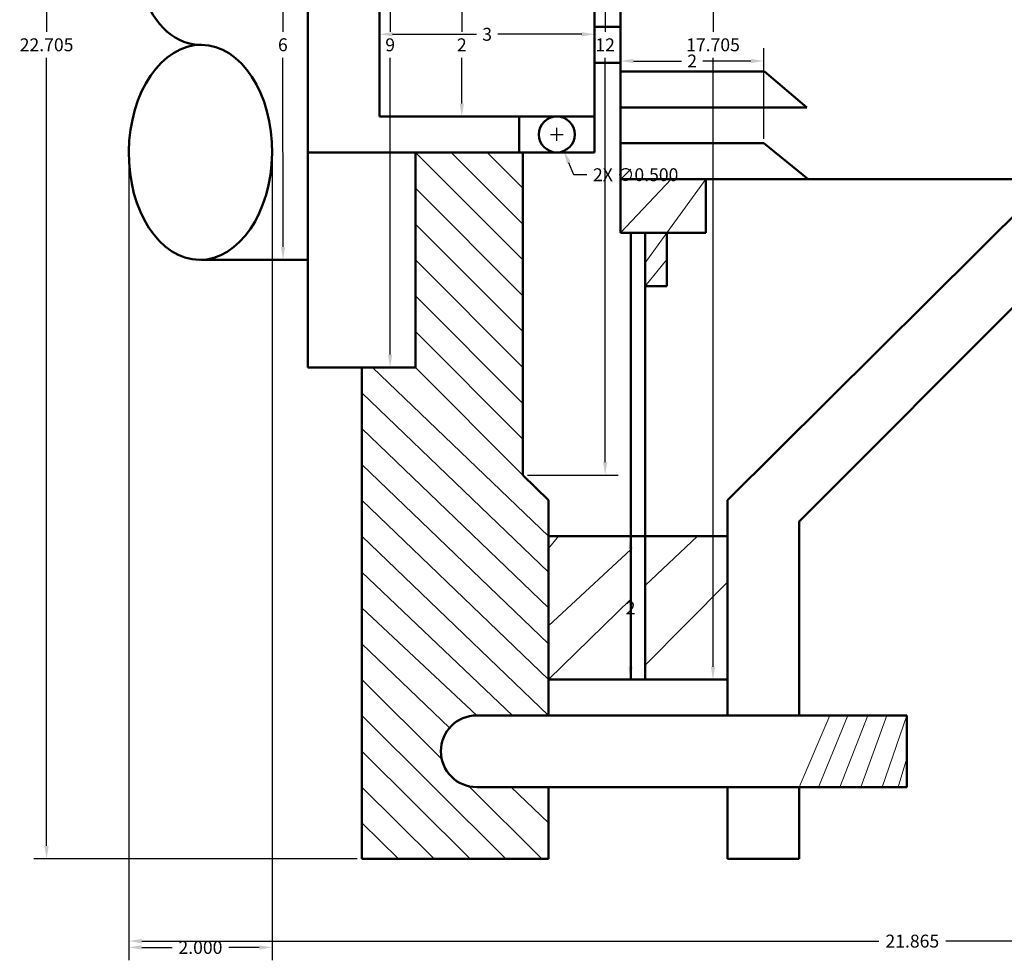
# Model space of a CAD drawing. Units: inches. Extents: x 15.4 to 41.1, y -0.4 to 25.1.
# Tile 1 of 4: x 16 to 29.7, y -0.4 to 12.7. Entities that reach past the tile are written whole.
import ezdxf

# ---------------------------------------------------------------- set-up
doc = ezdxf.new("R2010")
doc.units = ezdxf.units.IN
doc.header["$MEASUREMENT"] = 0
for name, color, linetype, lineweight in [('M-DIMS', 2, 'Continuous', 18), ('M-HATC', 8, 'Continuous', 18), ('M-OUTL', 7, 'Continuous', 50)]:
    doc.layers.add(name, color=color, linetype=linetype, lineweight=lineweight)
doc.styles.get("Standard").update_dxf_attribs({"font": 'arial.ttf'})
doc.dimstyles.get("Standard").update_dxf_attribs({"dimtxt": 0.18, "dimasz": 0.18, "dimexe": 0.18, "dimexo": 0.0625, "dimgap": 0.09, "dimtad": 0, "dimtih": 1, "dimtoh": 1, "dimdec": 4, "dimzin": 0, "dimdsep": 46, "dimtxsty": 'Standard', "dimcen": 0.09, "dimadec": 0, "dimazin": 0, "dimtfac": 1, "dimtdec": 4, "dimtofl": 0, "dimtmove": 0, "dimatfit": 3, "dimfxl": 1, "dimtolj": 1, "dimtzin": 0, "dimarcsym": 0})

# ---------------------------------------------------------------- blocks, each defined once
blk = doc.blocks.new('*D1')
at = {"layer": 'Defpoints', "color": 0, "transparency": 16777216}
for p in [(39.379, 12.649), (17.513, 10.885), (39.379, -0.125)]:
    blk.add_point(p, dxfattribs=at)
at = {"layer": 'M-DIMS', "color": 0, "lineweight": -2, "transparency": 16777216}
for p, q in [((39.379, 12.587), (39.379, -0.305)), ((17.513, 10.823), (17.513, -0.305)), ((17.693, -0.125), (27.98, -0.125)), ((39.199, -0.125), (28.912, -0.125))]:
    blk.add_line(p, q, dxfattribs=at)
at = {"layer": 'M-DIMS', "color": 0, "transparency": 16777216}
for points in [[(17.693, -0.095), (17.693, -0.155), (17.513, -0.125)], [(39.199, -0.095), (39.199, -0.155), (39.379, -0.125)]]:
    blk.add_solid(points, dxfattribs=at)
at = {"layer": 'M-DIMS', "color": 0, "transparency": 16777216, "insert": (28.446, -0.125), "char_height": 0.18, "attachment_point": 5}
blk.add_mtext('\\A1;21.865', dxfattribs=at)
blk = doc.blocks.new('*D2')
at = {"layer": 'Defpoints', "color": 0, "transparency": 16777216}
for p in [(16.366, 23.727), (20.763, 23.727), (20.763, 1.022)]:
    blk.add_point(p, dxfattribs=at)
at = {"layer": 'M-DIMS', "color": 0, "lineweight": -2, "transparency": 16777216}
for p, q in [((20.7, 23.727), (16.186, 23.727)), ((16.366, 23.547), (16.366, 12.557)), ((16.366, 1.202), (16.366, 12.193)), ((20.7, 1.022), (16.186, 1.022))]:
    blk.add_line(p, q, dxfattribs=at)
at = {"layer": 'M-DIMS', "color": 0, "transparency": 16777216}
for points in [[(16.336, 23.547), (16.396, 23.547), (16.366, 23.727)], [(16.336, 1.202), (16.396, 1.202), (16.366, 1.022)]]:
    blk.add_solid(points, dxfattribs=at)
at = {"layer": 'M-DIMS', "color": 0, "transparency": 16777216, "insert": (16.366, 12.375), "char_height": 0.18, "attachment_point": 5}
blk.add_mtext('\\A1;22.705', dxfattribs=at)
blk = doc.blocks.new('*D17')
at = {"layer": 'Defpoints', "color": 0, "transparency": 16777216}
for p in [(23.368, 5.522), (23.368, 3.522), (24.515, 3.522)]:
    blk.add_point(p, dxfattribs=at)
at = {"layer": 'M-DIMS', "color": 0, "lineweight": -2, "transparency": 16777216}
for p, q in [((23.43, 5.522), (24.695, 5.522)), ((24.515, 5.342), (24.515, 4.703)), ((24.515, 3.702), (24.515, 4.342)), ((23.43, 3.522), (24.695, 3.522))]:
    blk.add_line(p, q, dxfattribs=at)
at = {"layer": 'M-DIMS', "color": 0, "transparency": 16777216}
for points in [[(24.485, 5.342), (24.545, 5.342), (24.515, 5.522)], [(24.485, 3.702), (24.545, 3.702), (24.515, 3.522)]]:
    blk.add_solid(points, dxfattribs=at)
at = {"layer": 'M-DIMS', "color": 0, "transparency": 16777216, "insert": (24.515, 4.522), "char_height": 0.18, "attachment_point": 5}
blk.add_mtext('\\A1;2', dxfattribs=at)
blk = doc.blocks.new('*D18')
at = {"layer": 'Defpoints', "color": 0, "transparency": 16777216}
for p in [(24.518, 21.227), (24.518, 3.522), (25.665, 3.522)]:
    blk.add_point(p, dxfattribs=at)
at = {"layer": 'M-DIMS', "color": 0, "lineweight": -2, "transparency": 16777216}
for p, q in [((24.58, 21.227), (25.845, 21.227)), ((25.665, 21.047), (25.665, 12.557)), ((25.665, 3.702), (25.665, 12.193)), ((24.58, 3.522), (25.845, 3.522))]:
    blk.add_line(p, q, dxfattribs=at)
at = {"layer": 'M-DIMS', "color": 0, "transparency": 16777216}
for points in [[(25.635, 21.047), (25.695, 21.047), (25.665, 21.227)], [(25.635, 3.702), (25.695, 3.702), (25.665, 3.522)]]:
    blk.add_solid(points, dxfattribs=at)
at = {"layer": 'M-DIMS', "color": 0, "transparency": 16777216, "insert": (25.665, 12.375), "char_height": 0.18, "attachment_point": 5}
blk.add_mtext('\\A1;17.705', dxfattribs=at)
blk = doc.blocks.new('*D19')
at = {"layer": 'Defpoints', "color": 0, "transparency": 16777216}
for p in [(23.013, 18.375), (23.013, 6.375), (24.16, 6.375)]:
    blk.add_point(p, dxfattribs=at)
at = {"layer": 'M-DIMS', "color": 0, "lineweight": -2, "transparency": 16777216}
for p, q in [((23.075, 18.375), (24.34, 18.375)), ((24.16, 18.195), (24.16, 12.555)), ((24.16, 6.555), (24.16, 12.194)), ((23.075, 6.375), (24.34, 6.375))]:
    blk.add_line(p, q, dxfattribs=at)
at = {"layer": 'M-DIMS', "color": 0, "transparency": 16777216}
for points in [[(24.13, 18.195), (24.19, 18.195), (24.16, 18.375)], [(24.13, 6.555), (24.19, 6.555), (24.16, 6.375)]]:
    blk.add_solid(points, dxfattribs=at)
at = {"layer": 'M-DIMS', "color": 0, "transparency": 16777216, "insert": (24.16, 12.375), "char_height": 0.18, "attachment_point": 5}
blk.add_mtext('\\A1;12', dxfattribs=at)
blk = doc.blocks.new('*D21')
at = {"layer": 'Defpoints', "color": 0, "transparency": 16777216}
for p in [(20.013, 16.875), (20.013, 7.875), (21.16, 7.875)]:
    blk.add_point(p, dxfattribs=at)
at = {"layer": 'M-DIMS', "color": 0, "lineweight": -2, "transparency": 16777216}
for p, q in [((20.075, 16.875), (21.34, 16.875)), ((21.16, 16.695), (21.16, 12.557)), ((21.16, 8.055), (21.16, 12.193)), ((20.075, 7.875), (21.34, 7.875))]:
    blk.add_line(p, q, dxfattribs=at)
at = {"layer": 'M-DIMS', "color": 0, "transparency": 16777216}
for points in [[(21.13, 16.695), (21.19, 16.695), (21.16, 16.875)], [(21.13, 8.055), (21.19, 8.055), (21.16, 7.875)]]:
    blk.add_solid(points, dxfattribs=at)
at = {"layer": 'M-DIMS', "color": 0, "transparency": 16777216, "insert": (21.16, 12.375), "char_height": 0.18, "attachment_point": 5}
blk.add_mtext('\\A1;9', dxfattribs=at)
blk = doc.blocks.new('*D23')
at = {"layer": 'Defpoints', "color": 0, "transparency": 16777216}
for p in [(18.513, 15.375), (18.518, 9.375), (19.665, 9.376)]:
    blk.add_point(p, dxfattribs=at)
at = {"layer": 'M-DIMS', "color": 0, "lineweight": -2, "transparency": 16777216}
for p, q in [((18.575, 15.375), (19.84, 15.376)), ((19.66, 15.196), (19.663, 12.558)), ((19.665, 9.556), (19.663, 12.194)), ((18.58, 9.375), (19.845, 9.376))]:
    blk.add_line(p, q, dxfattribs=at)
at = {"layer": 'M-DIMS', "color": 0, "transparency": 16777216}
for points in [[(19.69, 15.196), (19.63, 15.196), (19.66, 15.376)], [(19.695, 9.556), (19.635, 9.556), (19.665, 9.376)]]:
    blk.add_solid(points, dxfattribs=at)
at = {"layer": 'M-DIMS', "color": 0, "transparency": 16777216, "insert": (19.663, 12.376), "char_height": 0.18, "attachment_point": 5}
blk.add_mtext('\\A1;6', dxfattribs=at)
blk = doc.blocks.new('*D24')
at = {"layer": 'Defpoints', "color": 0, "transparency": 16777216}
for p in [(21.013, 13.375), (21.013, 11.375), (22.16, 11.375)]:
    blk.add_point(p, dxfattribs=at)
at = {"layer": 'M-DIMS', "color": 0, "lineweight": -2, "transparency": 16777216}
for p, q in [((21.075, 13.375), (22.34, 13.375)), ((22.16, 13.195), (22.16, 12.555)), ((22.16, 11.555), (22.16, 12.194)), ((21.075, 11.375), (22.34, 11.375))]:
    blk.add_line(p, q, dxfattribs=at)
at = {"layer": 'M-DIMS', "color": 0, "transparency": 16777216}
for points in [[(22.13, 13.195), (22.19, 13.195), (22.16, 13.375)], [(22.13, 11.555), (22.19, 11.555), (22.16, 11.375)]]:
    blk.add_solid(points, dxfattribs=at)
at = {"layer": 'M-DIMS', "color": 0, "transparency": 16777216, "insert": (22.16, 12.375), "char_height": 0.18, "attachment_point": 5}
blk.add_mtext('\\A1;2', dxfattribs=at)
blk = doc.blocks.new('*D25')
at = {"layer": 'Defpoints', "color": 0, "transparency": 16777216}
for p in [(24.013, 12.522), (21.013, 11.375), (24.013, 11.375)]:
    blk.add_point(p, dxfattribs=at)
at = {"layer": 'M-DIMS', "color": 0, "lineweight": -2, "transparency": 16777216}
for p, q in [((21.013, 11.437), (21.013, 12.702)), ((24.013, 11.437), (24.013, 12.702)), ((21.193, 12.522), (22.364, 12.522)), ((23.833, 12.522), (22.662, 12.522))]:
    blk.add_line(p, q, dxfattribs=at)
at = {"layer": 'M-DIMS', "color": 0, "transparency": 16777216}
for points in [[(21.193, 12.552), (21.193, 12.492), (21.013, 12.522)], [(23.833, 12.552), (23.833, 12.492), (24.013, 12.522)]]:
    blk.add_solid(points, dxfattribs=at)
at = {"layer": 'M-DIMS', "color": 0, "transparency": 16777216, "insert": (22.513, 12.522), "char_height": 0.18, "attachment_point": 5}
blk.add_mtext('\\A1;3', dxfattribs=at)
blk = doc.blocks.new('*D30')
at = {"layer": 'Defpoints', "color": 0, "transparency": 16777216}
for p in [(26.374, 12.149), (24.374, 11.001), (26.374, 11.001)]:
    blk.add_point(p, dxfattribs=at)
at = {"layer": 'M-DIMS', "color": 0, "lineweight": -2, "transparency": 16777216}
for p, q in [((24.374, 11.064), (24.374, 12.329)), ((26.374, 11.064), (26.374, 12.329)), ((24.554, 12.149), (25.224, 12.149)), ((26.194, 12.149), (25.524, 12.149))]:
    blk.add_line(p, q, dxfattribs=at)
at = {"layer": 'M-DIMS', "color": 0, "transparency": 16777216}
for points in [[(24.554, 12.179), (24.554, 12.119), (24.374, 12.149)], [(26.194, 12.179), (26.194, 12.119), (26.374, 12.149)]]:
    blk.add_solid(points, dxfattribs=at)
at = {"layer": 'M-DIMS', "color": 0, "transparency": 16777216, "insert": (25.374, 12.149), "char_height": 0.18, "attachment_point": 5}
blk.add_mtext('\\A1;2', dxfattribs=at)
blk = doc.blocks.new('*D50')
at = {"layer": 'Defpoints', "color": 0, "transparency": 16777216}
for p in [(17.513, 10.885), (19.513, 10.864), (19.513, -0.213)]:
    blk.add_point(p, dxfattribs=at)
at = {"layer": 'M-DIMS', "color": 0, "lineweight": -2, "transparency": 16777216}
for p, q in [((17.513, 10.823), (17.513, -0.393)), ((19.513, 10.802), (19.513, -0.393)), ((17.693, -0.213), (18.118, -0.213)), ((19.333, -0.213), (18.908, -0.213))]:
    blk.add_line(p, q, dxfattribs=at)
at = {"layer": 'M-DIMS', "color": 0, "transparency": 16777216}
for points in [[(17.693, -0.183), (17.693, -0.243), (17.513, -0.213)], [(19.333, -0.183), (19.333, -0.243), (19.513, -0.213)]]:
    blk.add_solid(points, dxfattribs=at)
at = {"layer": 'M-DIMS', "color": 0, "transparency": 16777216, "insert": (18.513, -0.213), "char_height": 0.18, "attachment_point": 5}
blk.add_mtext('\\A1;2.000', dxfattribs=at)
blk = doc.blocks.new('*D60')
at = {"layer": 'Defpoints', "color": 0, "transparency": 16777216}
for p in [(23.388, 11.355), (23.584, 10.895)]:
    blk.add_point(p, dxfattribs=at)
at = {"layer": 'M-DIMS', "color": 0, "lineweight": -2, "transparency": 16777216}
for p, q in [((23.486, 11.035), (23.486, 11.215)), ((23.396, 11.125), (23.576, 11.125)), ((23.724, 10.563), (23.654, 10.729)), ((23.904, 10.563), (23.724, 10.563))]:
    blk.add_line(p, q, dxfattribs=at)
at = {"layer": 'M-DIMS', "color": 0, "transparency": 16777216}
blk.add_solid([(23.681, 10.741), (23.626, 10.717), (23.584, 10.895)], dxfattribs=at)
at = {"layer": 'M-DIMS', "color": 0, "transparency": 16777216, "insert": (24.586, 10.563), "char_height": 0.18, "attachment_point": 5}
blk.add_mtext('\\A1;2X ∅0.500', dxfattribs=at)

msp = doc.modelspace()

# ---------------------------------------------------------------- linework, layer by layer
at = {"layer": 'M-HATC'}
for p, q in [((23.0128, 9.3747), (21.5128, 10.8747)), ((22.0128, 10.8747), (23.0128, 9.8747)), ((22.5128, 10.8747), (23.0128, 10.3747)), ((24.374, 9.7512), (25.0794, 10.5012)), ((25.5651, 10.5012), (25.0198, 9.7512)), ((21.5128, 10.3747), (23.0128, 8.8747)), ((23.0128, 8.3747), (21.5128, 9.8747)), ((25.0198, 9.7512), (24.7176, 9.3356)), ((21.5128, 9.3747), (23.0128, 7.8747)), ((24.7176, 9.0071), (25.0198, 9.3792)), ((23.0128, 7.3747), (21.5128, 8.8747)), ((21.5128, 8.3747), (23.0128, 6.8747)), ((20.9128, 7.8747), (23.3676, 5.5224)), ((23.0128, 6.3747), (21.5128, 7.8747)), ((23.3676, 5.0224), (20.7628, 7.5224)), ((23.3676, 4.5224), (20.7628, 7.0224)), ((20.7628, 6.5224), (23.3676, 4.0224)), ((23.3676, 3.5224), (20.7628, 6.0224)), ((20.7628, 5.5224), (23.3676, 3.0224)), ((23.3676, 5.3495), (23.5085, 5.5224)), ((24.7176, 4.833), (25.4478, 5.5224)), ((23.3676, 4.2724), (24.5176, 5.3372)), ((22.8676, 3.0224), (20.7628, 5.0224)), ((24.7176, 3.7238), (25.8676, 4.8821)), ((23.3676, 3.5224), (24.5176, 4.6441)), ((22.3676, 3.0224), (20.7628, 4.5224)), ((20.7628, 4.0224), (21.9874, 2.8471)), ((21.8801, 2.411), (20.7628, 3.5224)), ((20.7628, 3.0224), (22.7762, 1.0224)), ((26.8676, 2.0224), (27.2933, 3.0224)), ((27.5483, 3.0224), (27.1388, 2.0224)), ((27.4324, 2.0224), (27.8264, 3.0224)), ((28.0892, 3.0224), (27.726, 2.0224)), ((28.0274, 2.0224), (28.3676, 3.0224)), ((22.2762, 1.0224), (20.7628, 2.5224)), ((28.2467, 2.0224), (28.3676, 2.4241)), ((20.7628, 2.0224), (21.7762, 1.0224)), ((23.2762, 1.0224), (22.2588, 2.0344)), ((22.8466, 2.0224), (23.3676, 1.5224)), ((20.7628, 1.5224), (21.2762, 1.0224))]:
    msp.add_line(p, q, dxfattribs=at)
at = {"layer": 'M-OUTL'}
for p, q in [((24.374, 10.5012), (24.374, 14.5012)), ((24.374, 10.5012), (24.374, 14.5012)), ((24.374, 14.2482), (24.374, 10.2482)), ((24.374, 14.2482), (24.374, 10.2482)), ((20.0128, 12.3747), (20.0128, 13.8747)), ((24.0128, 13.8747), (24.0128, 10.8747)), ((24.0128, 10.8747), (24.0128, 13.8747)), ((21.0128, 13.3747), (21.0128, 11.3747)), ((21.0128, 11.3747), (21.0128, 13.3747)), ((24.0128, 12.3747), (24.0128, 12.6247)), ((24.0128, 12.6247), (24.374, 12.6247)), ((18.513, 12.3747), (18.513, 12.3745)), ((18.5287, 12.3746), (18.513, 12.3746)), ((18.5287, 12.3746), (18.5287, 12.3753)), ((20.0128, 10.8747), (20.0128, 12.3747)), ((20.0128, 12.3747), (20.0128, 10.8747)), ((24.0128, 12.3747), (24.0128, 12.1247)), ((24.0128, 12.1247), (24.374, 12.1247)), ((24.374, 11.5012), (24.374, 12.0012)), ((24.374, 12.0012), (26.3813, 12.0012)), ((24.374, 11.5012), (24.374, 12.0012)), ((24.374, 12.0012), (26.3813, 12.0012)), ((26.3813, 12.0012), (26.9763, 11.5012)), ((26.3813, 12.0012), (26.9763, 11.5012)), ((24.374, 11.0012), (24.374, 11.5012)), ((24.374, 11.5012), (26.9763, 11.5012)), ((24.374, 11.0012), (24.374, 11.5012)), ((24.374, 11.5012), (26.9763, 11.5012)), ((21.0128, 11.3747), (24.0128, 11.3747)), ((24.0128, 11.3747), (21.0128, 11.3747)), ((22.9588, 11.3747), (22.9588, 10.8747)), ((22.9588, 10.8747), (22.9588, 11.3747)), ((22.9588, 11.3747), (24.0128, 11.3747)), ((24.0128, 10.8747), (24.0128, 11.3747)), ((24.0128, 10.8747), (24.0128, 11.3747)), ((24.374, 10.5012), (24.374, 11.0012)), ((24.374, 11.0012), (26.374, 11.0012)), ((24.374, 10.5012), (24.374, 11.0012)), ((24.374, 11.0012), (26.374, 11.0012)), ((26.374, 11.0012), (26.9908, 10.5012)), ((26.374, 11.0012), (26.9908, 10.5012)), ((24.0128, 10.8747), (20.0128, 10.8747)), ((20.0128, 7.8747), (20.0128, 10.8747)), ((20.0128, 10.8747), (20.0128, 7.8747)), ((20.0128, 10.8747), (24.0128, 10.8747)), ((24.0128, 10.8747), (20.0128, 10.8747)), ((20.0128, 10.8747), (20.0128, 7.8747)), ((21.5128, 10.8747), (21.5128, 7.8747)), ((21.5128, 7.8747), (21.5128, 10.8747)), ((21.5128, 7.8747), (21.5128, 10.8747)), ((21.5128, 10.8747), (23.0128, 10.8747)), ((21.5128, 10.3747), (21.5128, 10.8747)), ((21.5128, 10.8747), (22.0128, 10.8747)), ((22.0128, 10.8747), (22.5128, 10.8747)), ((23.0128, 10.8747), (23.0128, 6.8747)), ((23.0128, 10.8747), (23.0128, 6.8747)), ((30.124, 10.5012), (24.374, 10.5012)), ((24.374, 10.5012), (24.374, 9.7512)), ((30.124, 10.5012), (24.374, 10.5012)), ((24.374, 10.5012), (24.374, 9.7512)), ((25.0794, 10.5012), (25.5651, 10.5012)), ((25.5651, 9.7512), (25.5651, 10.5012)), ((25.5651, 9.7512), (25.5651, 10.5012)), ((21.5128, 9.8747), (21.5128, 10.3747)), ((21.5128, 9.8747), (21.5128, 10.3747)), ((23.0128, 9.8747), (23.0128, 10.3747)), ((25.8676, 6.0224), (30.124, 10.2512)), ((25.8676, 6.0224), (30.124, 10.2512)), ((26.8676, 5.7288), (31.1089, 9.9728)), ((26.8676, 5.7288), (31.1089, 9.9728)), ((21.5128, 9.3747), (21.5128, 9.8747)), ((23.0128, 9.3747), (23.0128, 9.8747)), ((24.374, 9.7512), (25.5651, 9.7512)), ((24.374, 9.7512), (25.5651, 9.7512)), ((24.5176, 9.2658), (24.5176, 9.7512)), ((24.5176, 9.2658), (24.5176, 9.7512)), ((24.7176, 9.1777), (24.7176, 9.7512)), ((24.7176, 9.1777), (24.7176, 9.7512)), ((25.0198, 9.0071), (25.0198, 9.7512)), ((25.0198, 9.0071), (25.0198, 9.7512)), ((18.518, 9.3749), (18.518, 9.3747)), ((18.518, 9.3747), (20.0128, 9.3747)), ((21.5128, 8.8747), (21.5128, 9.3747)), ((21.5128, 8.8747), (21.5128, 9.3747)), ((23.0128, 8.8747), (23.0128, 9.3747)), ((23.0128, 8.8747), (23.0128, 9.3747)), ((24.5176, 5.5224), (24.5176, 9.2658)), ((24.5176, 5.5224), (24.5176, 9.2658)), ((24.7176, 9.3356), (24.7176, 9.0071)), ((24.7176, 3.5224), (24.7176, 9.1777)), ((24.7176, 3.5224), (24.7176, 9.1777)), ((24.7176, 9.0071), (25.0198, 9.0071)), ((24.7176, 9.0071), (25.0198, 9.0071)), ((21.5128, 8.3747), (21.5128, 8.8747)), ((23.0128, 8.3747), (23.0128, 8.8747)), ((21.5128, 7.8747), (21.5128, 8.3747)), ((23.0128, 7.8747), (23.0128, 8.3747)), ((23.0128, 7.8747), (23.0128, 8.3747)), ((21.5128, 7.8747), (20.0128, 7.8747)), ((20.0128, 7.8747), (21.0128, 7.8747)), ((20.0128, 7.8747), (21.0128, 7.8747)), ((20.7628, 7.8747), (20.7628, 1.0224)), ((20.7628, 7.8747), (20.7628, 1.0224)), ((20.7628, 7.5224), (20.7628, 7.8747)), ((20.7628, 7.8747), (20.9128, 7.8747)), ((21.0128, 7.8747), (21.5128, 7.8747)), ((21.0128, 7.8747), (21.5128, 7.8747)), ((23.0128, 7.3747), (23.0128, 7.8747)), ((20.7628, 7.0224), (20.7628, 7.5224)), ((20.7628, 7.0224), (20.7628, 7.5224)), ((23.0128, 6.8747), (23.0128, 7.3747)), ((23.0128, 6.8747), (23.0128, 7.3747)), ((20.7628, 6.5224), (20.7628, 7.0224)), ((23.0128, 6.8747), (23.0128, 6.3747)), ((23.0128, 6.8747), (23.0128, 6.3747)), ((23.0128, 6.3747), (23.0128, 6.8747)), ((20.7628, 6.0224), (20.7628, 6.5224)), ((20.7628, 6.0224), (20.7628, 6.5224)), ((23.0128, 6.3747), (23.3676, 6.0224)), ((23.0128, 6.3747), (23.3676, 6.0224)), ((20.7628, 5.5224), (20.7628, 6.0224)), ((23.3676, 6.0224), (23.3676, 3.0224)), ((23.3676, 6.0224), (23.3676, 3.0224)), ((23.3676, 6.0224), (23.3676, 5.5224)), ((25.8676, 3.0224), (25.8676, 6.0224)), ((25.8676, 3.0224), (25.8676, 6.0224)), ((26.8676, 3.0224), (26.8676, 5.7288)), ((26.8676, 3.0224), (26.8676, 5.7288)), ((20.7628, 5.0224), (20.7628, 5.5224)), ((23.3676, 5.5224), (25.8676, 5.5224)), ((23.3676, 5.5224), (25.8676, 5.5224)), ((23.3676, 5.5224), (23.3676, 4.7724)), ((24.5176, 3.5224), (24.5176, 5.5224)), ((24.5176, 3.5224), (24.5176, 5.5224)), ((20.7628, 4.5224), (20.7628, 5.0224)), ((23.3676, 4.5224), (23.3676, 5.0224)), ((20.7628, 4.0224), (20.7628, 4.5224)), ((23.3676, 4.0224), (23.3676, 4.5224)), ((20.7628, 3.5224), (20.7628, 4.0224)), ((23.3676, 3.0224), (23.3676, 4.0224)), ((20.7628, 3.0224), (20.7628, 3.5224)), ((23.3676, 3.5224), (25.8676, 3.5224)), ((23.3676, 3.5224), (24.5176, 3.5224)), ((23.3676, 3.0224), (23.3676, 3.5224)), ((23.3676, 3.5224), (25.8676, 3.5224)), ((23.3676, 3.5224), (24.5176, 3.5224)), ((23.3676, 3.0224), (23.3676, 3.5224)), ((25.8676, 3.5224), (24.7176, 3.5224)), ((25.8676, 3.5224), (24.7176, 3.5224)), ((20.7628, 2.5224), (20.7628, 3.0224)), ((20.7628, 2.5224), (20.7628, 3.0224)), ((23.3676, 3.0224), (22.3676, 3.0224)), ((23.3676, 3.0224), (22.3676, 3.0224)), ((22.3676, 3.0224), (22.8676, 3.0224)), ((28.3676, 3.0224), (23.3676, 3.0224)), ((28.3676, 3.0224), (23.3676, 3.0224)), ((27.2933, 3.0224), (27.5483, 3.0224)), ((27.8264, 3.0224), (28.0892, 3.0224)), ((28.3676, 2.0224), (28.3676, 3.0224)), ((28.3676, 2.0224), (28.3676, 3.0224)), ((28.3676, 3.0224), (28.3676, 2.4241)), ((20.7628, 2.0224), (20.7628, 2.5224)), ((20.7628, 1.5224), (20.7628, 2.0224)), ((22.3676, 2.0224), (23.3676, 2.0224)), ((22.3676, 2.0224), (23.3676, 2.0224)), ((23.3676, 2.0224), (23.3676, 1.0224)), ((23.3676, 2.0224), (28.3676, 2.0224)), ((23.3676, 2.0224), (23.3676, 1.0224)), ((23.3676, 2.0224), (28.3676, 2.0224)), ((25.8676, 2.0224), (25.8676, 1.0224)), ((25.8676, 2.0224), (25.8676, 1.0224)), ((26.8676, 1.0224), (26.8676, 2.0224)), ((26.8676, 1.0224), (26.8676, 2.0224)), ((27.1388, 2.0224), (27.4324, 2.0224)), ((27.726, 2.0224), (28.0274, 2.0224)), ((28.0274, 2.0224), (28.2467, 2.0224)), ((20.7628, 1.0224), (20.7628, 1.5224)), ((23.3676, 1.0224), (23.3676, 1.5224)), ((23.3676, 1.0224), (20.7628, 1.0224)), ((23.3676, 1.0224), (20.7628, 1.0224)), ((21.2762, 1.0224), (21.7762, 1.0224)), ((21.7762, 1.0224), (22.2762, 1.0224)), ((21.7762, 1.0224), (22.2762, 1.0224)), ((22.2762, 1.0224), (22.7762, 1.0224)), ((22.7762, 1.0224), (23.2762, 1.0224)), ((22.7762, 1.0224), (23.2762, 1.0224)), ((25.8676, 1.0224), (26.8676, 1.0224)), ((25.8676, 1.0224), (26.8676, 1.0224))]:
    msp.add_line(p, q, dxfattribs=at)
msp.add_circle((23.4858, 11.1247), 0.25, dxfattribs=at)
msp.add_circle((23.4858, 11.1247), 0.25, dxfattribs=at)
for centre, radius, start, end in [((18.5129, 13.8747), 1.5002, 269.15251, 270.60328), ((18.5131, 10.8747), 1.5, 89.40474, 90.60336), ((18.5131, 10.8747), 1.5, 358.86538, 1.13462), ((22.3676, 2.5224), 0.5, 90, 270)]:
    msp.add_arc(centre, radius, start, end, dxfattribs=at)
msp.add_ellipse((18.5129, 13.8747), major_axis=(0.0222, 1.5), ratio=0.6275384, start_param=0, end_param=3.1819287, dxfattribs=at)
msp.add_ellipse((18.5131, 10.8747), major_axis=(0.0156, 1.4999), ratio=0.6666694, dxfattribs=at)

# ---------------------------------------------------------------- dimensions: what is measured, and where the dimension line sits
at = {"layer": 'M-DIMS'}
for base, p1, p2, angle, override, picture, middle in [((16.3657, 23.727), (20.7628, 1.0224), (20.7628, 23.727), 90, {"dimdec": 3, "dimlfac": 1, "dimrnd": 0, "dimzin": 0, "dimdsep": 46, "dimlunit": 2}, '*D2', (16.3657, 12.3747)), ((25.6651, 3.5224), (24.5176, 21.227), (24.5176, 3.5224), 270, {"dimdec": 3, "dimlfac": 1, "dimrnd": 0, "dimzin": 0, "dimdsep": 46, "dimlunit": 2}, '*D18', (25.6651, 12.3747)), ((24.1603, 6.3747), (23.0128, 18.3747), (23.0128, 6.3747), 270, {"dimdec": 0, "dimlfac": 1, "dimrnd": 0, "dimzin": 0, "dimdsep": 46, "dimlunit": 2}, '*D19', (24.1603, 12.3747)), ((21.1603, 7.8747), (20.0128, 16.8747), (20.0128, 7.8747), 270, {"dimdec": 0, "dimlfac": 1, "dimrnd": 0, "dimzin": 0, "dimdsep": 46, "dimlunit": 2}, '*D21', (21.1603, 12.3747)), ((19.6655, 9.3757), (18.5128, 15.3747), (18.518, 9.3747), 270.0497, {"dimdec": 0, "dimlfac": 1, "dimrnd": 0, "dimzin": 0, "dimdsep": 46, "dimlunit": 2}, '*D23', (19.6629, 12.3757)), ((22.1603, 11.3747), (21.0128, 13.3747), (21.0128, 11.3747), 270, {"dimdec": 0, "dimlfac": 1, "dimrnd": 0, "dimzin": 0, "dimdsep": 46, "dimlunit": 2}, '*D24', (22.1603, 12.3747)), ((24.5151, 3.5224), (23.3676, 5.5224), (23.3676, 3.5224), 270, {"dimdec": 0, "dimlfac": 1, "dimrnd": 0, "dimzin": 0, "dimdsep": 46, "dimlunit": 2}, '*D17', (24.5151, 4.5224))]:
    dim = msp.add_linear_dim(base=base, p1=p1, p2=p2, angle=angle, dimstyle='Standard', override=override, dxfattribs=at)
    dim.commit()
    dim.dimension.update_dxf_attribs({"geometry": picture, "text_midpoint": middle})
for base, p1, p2, override, picture, middle in [((39.3785, -0.1251), (17.5132, 10.8851), (39.3785, 12.6491), {"dimdec": 3, "dimlfac": 1, "dimrnd": 0, "dimzin": 0, "dimdsep": 46, "dimlunit": 2}, '*D1', (28.4458, -0.1251)), ((24.0128, 12.5222), (21.0128, 11.3747), (24.0128, 11.3747), {"dimdec": 0, "dimlfac": 1, "dimrnd": 0, "dimzin": 0, "dimdsep": 46, "dimlunit": 2}, '*D25', (22.5128, 12.5222)), ((26.374, 12.1487), (24.374, 11.0012), (26.374, 11.0012), {"dimdec": 0, "dimlfac": 1, "dimrnd": 0, "dimzin": 0, "dimdsep": 46, "dimlunit": 2}, '*D30', (25.374, 12.1487)), ((19.513, -0.2126), (17.5132, 10.8851), (19.513, 10.8643), {"dimdec": 3, "dimlfac": 1, "dimrnd": 0, "dimzin": 0, "dimdsep": 46, "dimlunit": 2}, '*D50', (18.5131, -0.2126))]:
    dim = msp.add_linear_dim(base=base, p1=p1, p2=p2, dimstyle='Standard', override=override, dxfattribs=at)
    dim.commit()
    dim.dimension.update_dxf_attribs({"geometry": picture, "text_midpoint": middle})
dim = msp.add_diameter_dim_2p(p1=(23.3881, 11.3548), p2=(23.5835, 10.8946), text='2X <>', dimstyle='Standard', override={"dimdec": 3, "dimlfac": 1, "dimrnd": 0, "dimzin": 0, "dimdsep": 46, "dimlunit": 2}, dxfattribs=at)
dim.commit()
dim.dimension.update_dxf_attribs({"geometry": '*D60', "text_midpoint": (24.5857, 10.5632), "dimtype": 163})

doc.saveas('drawing.dxf')
